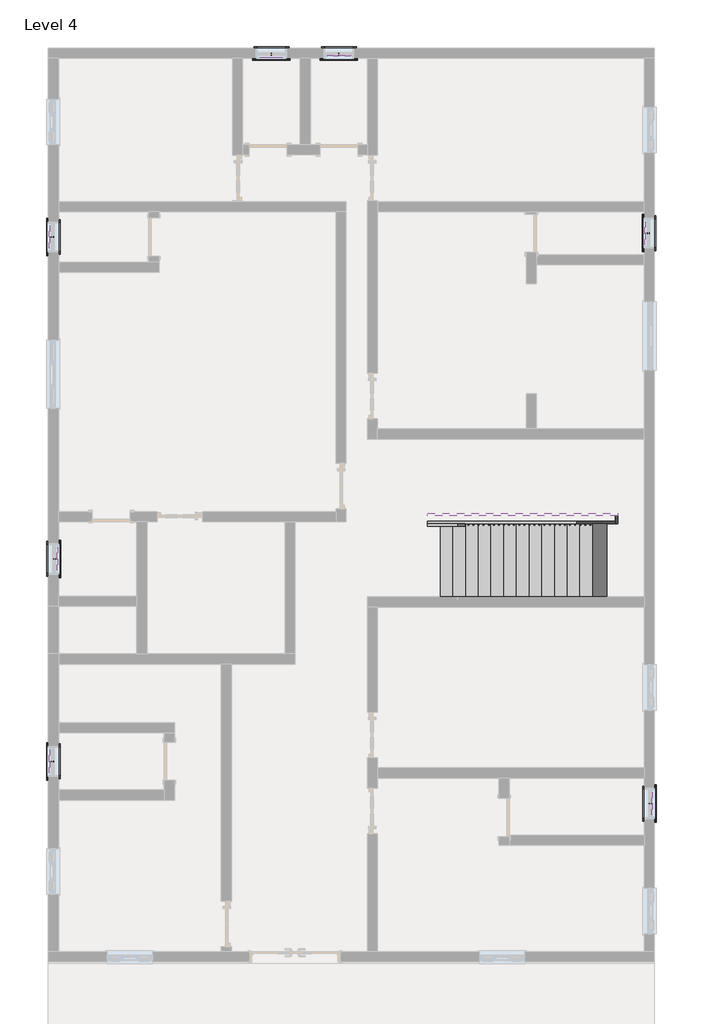
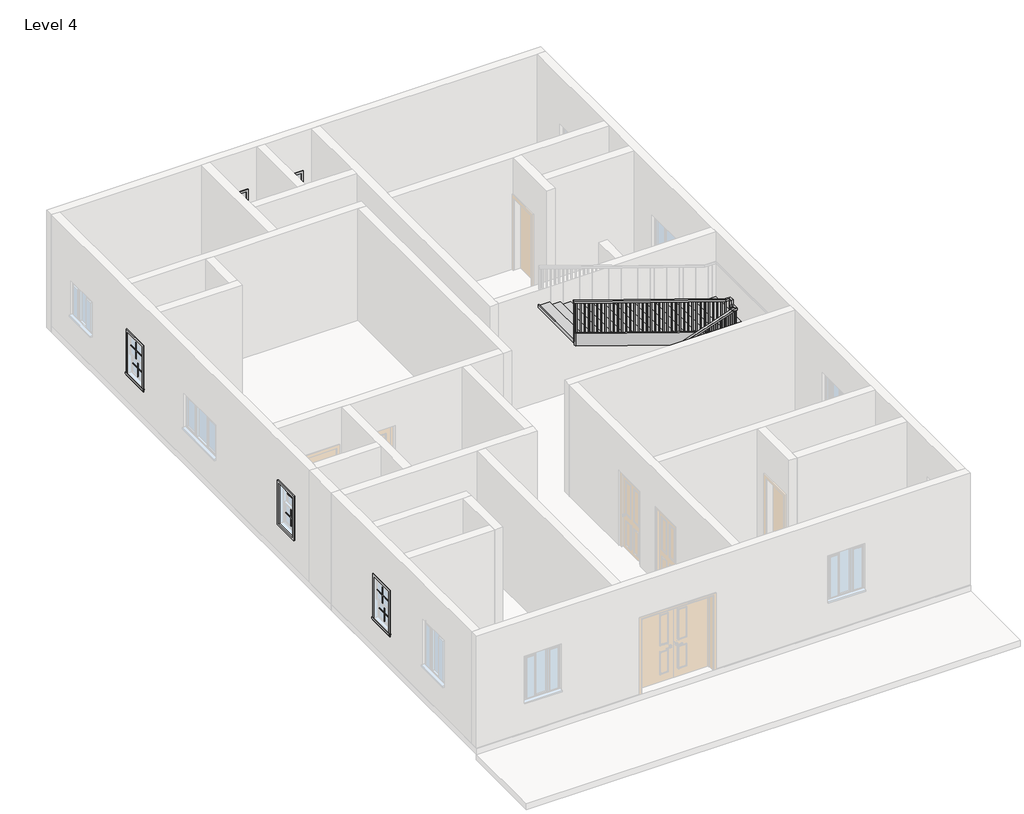
# One storey, part 3 of 3: 28 proxies, 6 members, 1 railing, 1 stair flight.
"""IFC4 building model written with IfcOpenShell, lengths in millimetres."""

from ifc_helpers import new_model, si_unit, frame, origin, place, context, project, spatial, polyline, outline, extrude, faceted_brep, transform, mapped, element, save
from components import muntin_pattern_2x2_muntin_pattern_2x2_eba6c5fb, trim_window_exterior_flat_with_sill_278e6a94, trim_window_interior_flat_picture_frame_e9fd5f45, stair_flight_fd3cf4e0

model = new_model("IFC4")

# Units and contexts
model_context = context("Model", 3, world=origin())
ifc_project = project(units=[si_unit("LENGTHUNIT", "METRE", prefix="MILLI")], contexts=[model_context])

# Site, building, storey
site = spatial("IfcSite", under=ifc_project)
building = spatial("IfcBuilding", under=site)
storey = spatial("IfcBuildingStorey", under=building, Name="Level 4", Elevation=9144.0)

# Proxies
placement = place(None, origin())
muntin_pattern_2x2_muntin_pattern_2x2_shape = muntin_pattern_2x2_muntin_pattern_2x2_eba6c5fb(model_context)
element("IfcBuildingElementProxy", 1, Name="Muntin Pattern_2x2 : Muntin Pattern_2x2", ObjectType="Muntin Pattern_2x2 : Muntin Pattern_2x2", at=placement, inside=storey, context=model_context, shape_type="MappedRepresentation", body=[
    mapped(muntin_pattern_2x2_muntin_pattern_2x2_shape, transform((-6096.8589448, 5183.1303322, 10614.025), x_axis=(0.0, 1.0, 0.0), y_axis=(-1.0, 0.0, 0.0), z_axis=(0.0, 0.0, 1.0))),
])
element("IfcBuildingElementProxy", 2, Name="Muntin Pattern_2x2 : Muntin Pattern_2x2", ObjectType="Muntin Pattern_2x2 : Muntin Pattern_2x2", at=placement, inside=storey, context=model_context, shape_type="MappedRepresentation", body=[
    mapped(muntin_pattern_2x2_muntin_pattern_2x2_shape, transform((-6052.4089448, 5183.1303322, 10134.6), x_axis=(0.0, 1.0, 0.0), y_axis=(-1.0, 0.0, 0.0), z_axis=(0.0, 0.0, 1.0))),
])
element("IfcBuildingElementProxy", 3, Name="Muntin Pattern_2x2 : Muntin Pattern_2x2", ObjectType="Muntin Pattern_2x2 : Muntin Pattern_2x2", at=placement, inside=storey, context=model_context, shape_type="MappedRepresentation", body=[
    mapped(muntin_pattern_2x2_muntin_pattern_2x2_shape, transform((-1673.5309118, 8787.5224079, 10614.025), x_axis=(-1.0, 0.0, 0.0), y_axis=(0.0, -1.0, 0.0), z_axis=(0.0, 0.0, 1.0))),
])
element("IfcBuildingElementProxy", 4, Name="Muntin Pattern_2x2 : Muntin Pattern_2x2", ObjectType="Muntin Pattern_2x2 : Muntin Pattern_2x2", at=placement, inside=storey, context=model_context, shape_type="MappedRepresentation", body=[
    mapped(muntin_pattern_2x2_muntin_pattern_2x2_shape, transform((-1673.5309118, 8831.9724079, 10134.6), x_axis=(-1.0, 0.0, 0.0), y_axis=(0.0, -1.0, 0.0), z_axis=(0.0, 0.0, 1.0))),
])
element("IfcBuildingElementProxy", 5, Name="Muntin Pattern_2x2 : Muntin Pattern_2x2", ObjectType="Muntin Pattern_2x2 : Muntin Pattern_2x2", at=placement, inside=storey, context=model_context, shape_type="MappedRepresentation", body=[
    mapped(muntin_pattern_2x2_muntin_pattern_2x2_shape, transform((-324.5451949, 8787.5224079, 10614.025), x_axis=(-1.0, 0.0, 0.0), y_axis=(0.0, -1.0, 0.0), z_axis=(0.0, 0.0, 1.0))),
])
element("IfcBuildingElementProxy", 6, Name="Muntin Pattern_2x2 : Muntin Pattern_2x2", ObjectType="Muntin Pattern_2x2 : Muntin Pattern_2x2", at=placement, inside=storey, context=model_context, shape_type="MappedRepresentation", body=[
    mapped(muntin_pattern_2x2_muntin_pattern_2x2_shape, transform((-324.5451949, 8831.9724079, 10134.6), x_axis=(-1.0, 0.0, 0.0), y_axis=(0.0, -1.0, 0.0), z_axis=(0.0, 0.0, 1.0))),
])
element("IfcBuildingElementProxy", 7, Name="Muntin Pattern_2x2 : Muntin Pattern_2x2", ObjectType="Muntin Pattern_2x2 : Muntin Pattern_2x2", at=placement, inside=storey, context=model_context, shape_type="MappedRepresentation", body=[
    mapped(muntin_pattern_2x2_muntin_pattern_2x2_shape, transform((5813.4689795, 5259.3303322, 10614.025), x_axis=(0.0, 1.0, 0.0), y_axis=(-1.0, 0.0, 0.0), z_axis=(0.0, 0.0, 1.0))),
])
element("IfcBuildingElementProxy", 8, Name="Muntin Pattern_2x2 : Muntin Pattern_2x2", ObjectType="Muntin Pattern_2x2 : Muntin Pattern_2x2", at=placement, inside=storey, context=model_context, shape_type="MappedRepresentation", body=[
    mapped(muntin_pattern_2x2_muntin_pattern_2x2_shape, transform((5857.9189795, 5259.3303322, 10134.6), x_axis=(0.0, 1.0, 0.0), y_axis=(-1.0, 0.0, 0.0), z_axis=(0.0, 0.0, 1.0))),
])
element("IfcBuildingElementProxy", 9, Name="Muntin Pattern_2x2 : Muntin Pattern_2x2", ObjectType="Muntin Pattern_2x2 : Muntin Pattern_2x2", at=placement, inside=storey, context=model_context, shape_type="MappedRepresentation", body=[
    mapped(muntin_pattern_2x2_muntin_pattern_2x2_shape, transform((5946.8189795, -6133.2488489, 10614.025), x_axis=(0.0, -1.0, 0.0), y_axis=(1.0, 0.0, 0.0), z_axis=(0.0, 0.0, 1.0))),
])
element("IfcBuildingElementProxy", 10, Name="Muntin Pattern_2x2 : Muntin Pattern_2x2", ObjectType="Muntin Pattern_2x2 : Muntin Pattern_2x2", at=placement, inside=storey, context=model_context, shape_type="MappedRepresentation", body=[
    mapped(muntin_pattern_2x2_muntin_pattern_2x2_shape, transform((5902.3689795, -6133.2488489, 10134.6), x_axis=(0.0, -1.0, 0.0), y_axis=(1.0, 0.0, 0.0), z_axis=(0.0, 0.0, 1.0))),
])
element("IfcBuildingElementProxy", 11, Name="Muntin Pattern_2x2 : Muntin Pattern_2x2", ObjectType="Muntin Pattern_2x2 : Muntin Pattern_2x2", at=placement, inside=storey, context=model_context, shape_type="MappedRepresentation", body=[
    mapped(muntin_pattern_2x2_muntin_pattern_2x2_shape, transform((-6096.8589448, -5291.0659014, 10614.025), x_axis=(0.0, 1.0, 0.0), y_axis=(-1.0, 0.0, 0.0), z_axis=(0.0, 0.0, 1.0))),
])
element("IfcBuildingElementProxy", 12, Name="Muntin Pattern_2x2 : Muntin Pattern_2x2", ObjectType="Muntin Pattern_2x2 : Muntin Pattern_2x2", at=placement, inside=storey, context=model_context, shape_type="MappedRepresentation", body=[
    mapped(muntin_pattern_2x2_muntin_pattern_2x2_shape, transform((-6052.4089448, -5291.0659014, 10134.6), x_axis=(0.0, 1.0, 0.0), y_axis=(-1.0, 0.0, 0.0), z_axis=(0.0, 0.0, 1.0))),
])
element("IfcBuildingElementProxy", 13, Name="Muntin Pattern_2x2 : Muntin Pattern_2x2", ObjectType="Muntin Pattern_2x2 : Muntin Pattern_2x2", at=placement, inside=storey, context=model_context, shape_type="MappedRepresentation", body=[
    mapped(muntin_pattern_2x2_muntin_pattern_2x2_shape, transform((-5963.5089448, -1246.1159014, 10614.025), x_axis=(0.0, -1.0, 0.0), y_axis=(1.0, 0.0, 0.0), z_axis=(0.0, 0.0, 1.0))),
])
element("IfcBuildingElementProxy", 14, Name="Muntin Pattern_2x2 : Muntin Pattern_2x2", ObjectType="Muntin Pattern_2x2 : Muntin Pattern_2x2", at=placement, inside=storey, context=model_context, shape_type="MappedRepresentation", body=[
    mapped(muntin_pattern_2x2_muntin_pattern_2x2_shape, transform((-6007.9589448, -1246.1159014, 10134.6), x_axis=(0.0, -1.0, 0.0), y_axis=(1.0, 0.0, 0.0), z_axis=(0.0, 0.0, 1.0))),
])
trim_window_exterior_flat_with_sill_shape = trim_window_exterior_flat_with_sill_278e6a94(model_context)
element("IfcBuildingElementProxy", 15, Name="Trim-Window-Exterior-Flat : with Sill", ObjectType="Trim-Window-Exterior-Flat : with Sill", at=placement, inside=storey, context=model_context, shape_type="MappedRepresentation", body=[
    mapped(trim_window_exterior_flat_with_sill_shape, transform((-6131.7839448, 5183.1303322, 11125.2), x_axis=(0.0, -1.0, 0.0), y_axis=(0.0, 0.0, 1.0), z_axis=(-1.0, 0.0, 0.0))),
])
element("IfcBuildingElementProxy", 16, Name="Trim-Window-Exterior-Flat : with Sill", ObjectType="Trim-Window-Exterior-Flat : with Sill", at=placement, inside=storey, context=model_context, shape_type="MappedRepresentation", body=[
    mapped(trim_window_exterior_flat_with_sill_shape, transform((-1673.5309118, 8752.5974079, 11125.2), x_axis=(1.0, 0.0, 0.0), y_axis=(0.0, 0.0, 1.0), z_axis=(0.0, -1.0, 0.0))),
])
element("IfcBuildingElementProxy", 17, Name="Trim-Window-Exterior-Flat : with Sill", ObjectType="Trim-Window-Exterior-Flat : with Sill", at=placement, inside=storey, context=model_context, shape_type="MappedRepresentation", body=[
    mapped(trim_window_exterior_flat_with_sill_shape, transform((-324.5451949, 8752.5974079, 11125.2), x_axis=(1.0, 0.0, 0.0), y_axis=(0.0, 0.0, 1.0), z_axis=(0.0, -1.0, 0.0))),
])
element("IfcBuildingElementProxy", 18, Name="Trim-Window-Exterior-Flat : with Sill", ObjectType="Trim-Window-Exterior-Flat : with Sill", at=placement, inside=storey, context=model_context, shape_type="MappedRepresentation", body=[
    mapped(trim_window_exterior_flat_with_sill_shape, transform((5778.5439795, 5259.3303322, 11125.2), x_axis=(0.0, -1.0, 0.0), y_axis=(0.0, 0.0, 1.0), z_axis=(-1.0, 0.0, 0.0))),
])
element("IfcBuildingElementProxy", 19, Name="Trim-Window-Exterior-Flat : with Sill", ObjectType="Trim-Window-Exterior-Flat : with Sill", at=placement, inside=storey, context=model_context, shape_type="MappedRepresentation", body=[
    mapped(trim_window_exterior_flat_with_sill_shape, transform((5981.7439795, -6133.2488489, 11125.2), x_axis=(0.0, 1.0, 0.0), y_axis=(0.0, 0.0, 1.0), z_axis=(1.0, 0.0, 0.0))),
])
element("IfcBuildingElementProxy", 20, Name="Trim-Window-Exterior-Flat : with Sill", ObjectType="Trim-Window-Exterior-Flat : with Sill", at=placement, inside=storey, context=model_context, shape_type="MappedRepresentation", body=[
    mapped(trim_window_exterior_flat_with_sill_shape, transform((-6131.7839448, -5291.0659014, 11125.2), x_axis=(0.0, -1.0, 0.0), y_axis=(0.0, 0.0, 1.0), z_axis=(-1.0, 0.0, 0.0))),
])
element("IfcBuildingElementProxy", 21, Name="Trim-Window-Exterior-Flat : with Sill", ObjectType="Trim-Window-Exterior-Flat : with Sill", at=placement, inside=storey, context=model_context, shape_type="MappedRepresentation", body=[
    mapped(trim_window_exterior_flat_with_sill_shape, transform((-5928.5839448, -1246.1159014, 11125.2), x_axis=(0.0, 1.0, 0.0), y_axis=(0.0, 0.0, 1.0), z_axis=(1.0, 0.0, 0.0))),
])
trim_window_interior_flat_picture_frame_shape = trim_window_interior_flat_picture_frame_e9fd5f45(model_context)
element("IfcBuildingElementProxy", 22, Name="Trim-Window-Interior-Flat : Picture Frame", ObjectType="Trim-Window-Interior-Flat : Picture Frame", at=placement, inside=storey, context=model_context, shape_type="MappedRepresentation", body=[
    mapped(trim_window_interior_flat_picture_frame_shape, transform((-5928.5839448, 5183.1303322, 11125.2), x_axis=(0.0, 1.0, 0.0), y_axis=(0.0, 0.0, 1.0), z_axis=(1.0, 0.0, 0.0))),
])
element("IfcBuildingElementProxy", 23, Name="Trim-Window-Interior-Flat : Picture Frame", ObjectType="Trim-Window-Interior-Flat : Picture Frame", at=placement, inside=storey, context=model_context, shape_type="MappedRepresentation", body=[
    mapped(trim_window_interior_flat_picture_frame_shape, transform((-1673.5309118, 8955.7974079, 11125.2), x_axis=(-1.0, 0.0, 0.0), y_axis=(0.0, 0.0, 1.0), z_axis=(0.0, 1.0, 0.0))),
])
element("IfcBuildingElementProxy", 24, Name="Trim-Window-Interior-Flat : Picture Frame", ObjectType="Trim-Window-Interior-Flat : Picture Frame", at=placement, inside=storey, context=model_context, shape_type="MappedRepresentation", body=[
    mapped(trim_window_interior_flat_picture_frame_shape, transform((-324.5451949, 8955.7974079, 11125.2), x_axis=(-1.0, 0.0, 0.0), y_axis=(0.0, 0.0, 1.0), z_axis=(0.0, 1.0, 0.0))),
])
element("IfcBuildingElementProxy", 25, Name="Trim-Window-Interior-Flat : Picture Frame", ObjectType="Trim-Window-Interior-Flat : Picture Frame", at=placement, inside=storey, context=model_context, shape_type="MappedRepresentation", body=[
    mapped(trim_window_interior_flat_picture_frame_shape, transform((5981.7439795, 5259.3303322, 11125.2), x_axis=(0.0, 1.0, 0.0), y_axis=(0.0, 0.0, 1.0), z_axis=(1.0, 0.0, 0.0))),
])
element("IfcBuildingElementProxy", 26, Name="Trim-Window-Interior-Flat : Picture Frame", ObjectType="Trim-Window-Interior-Flat : Picture Frame", at=placement, inside=storey, context=model_context, shape_type="MappedRepresentation", body=[
    mapped(trim_window_interior_flat_picture_frame_shape, transform((5778.5439795, -6133.2488489, 11125.2), x_axis=(0.0, -1.0, 0.0), y_axis=(0.0, 0.0, 1.0), z_axis=(-1.0, 0.0, 0.0))),
])
element("IfcBuildingElementProxy", 27, Name="Trim-Window-Interior-Flat : Picture Frame", ObjectType="Trim-Window-Interior-Flat : Picture Frame", at=placement, inside=storey, context=model_context, shape_type="MappedRepresentation", body=[
    mapped(trim_window_interior_flat_picture_frame_shape, transform((-5928.5839448, -5291.0659014, 11125.2), x_axis=(0.0, 1.0, 0.0), y_axis=(0.0, 0.0, 1.0), z_axis=(1.0, 0.0, 0.0))),
])
element("IfcBuildingElementProxy", 28, Name="Trim-Window-Interior-Flat : Picture Frame", ObjectType="Trim-Window-Interior-Flat : Picture Frame", at=placement, inside=storey, context=model_context, shape_type="MappedRepresentation", body=[
    mapped(trim_window_interior_flat_picture_frame_shape, transform((-6131.7839448, -1246.1159014, 11125.2), x_axis=(0.0, -1.0, 0.0), y_axis=(0.0, 0.0, 1.0), z_axis=(-1.0, 0.0, 0.0))),
])

# Members
element("IfcMember", 29, ObjectType="Stringer - 2\" Width", at=placement, inside=storey, context=model_context, shape_type="SweptSolid", body=[
    extrude(outline(polyline([(9337.7751932, 1449.3932247), (9144.0, 1449.3932247), (9144.0, 1827.5890963), (10284.094539, 5195.8669505), (10591.8, 5195.8669505), (10591.8, 5154.2649181), (9337.7751932, 1449.3932247)])), frame((0.0, -541.2659014, 0.0), z_axis=(0.0, 1.0, 0.0), x_axis=(0.0, 0.0, 1.0)), (0.0, 0.0, 1.0), 50.8),
])
element("IfcMember", 30, ObjectType="Stringer - 2\" Width", at=placement, inside=storey, context=model_context, shape_type="SweptSolid", body=[
    extrude(outline(polyline([(5246.6669505, -541.2659014), (5195.8669505, -541.2659014), (5195.8669505, -388.7910016), (5246.6669505, -388.7910016), (5246.6669505, -541.2659014)])), frame((0.0, 0.0, 10287.0), z_axis=(0.0, 0.0, 1.0), x_axis=(1.0, 0.0, 0.0)), (0.0, 0.0, 1.0), 304.8),
])
element("IfcMember", 31, ObjectType="Stringer - 2\" Width", at=placement, inside=storey, context=model_context, shape_type="SweptSolid", body=[
    extrude(outline(polyline([(10387.0143208, 5246.6669505), (10708.8012358, 5246.6669505), (11994.1022784, 1449.3932247), (11672.3153634, 1449.3932247), (10387.0143208, 5246.6669505)])), frame((0.0, -388.7910016, 0.0), z_axis=(0.0, 1.0, 0.0), x_axis=(0.0, 0.0, 1.0)), (0.0, 0.0, 1.0), 50.8),
])
element("IfcMember", 32, ObjectType="Stringer - 2\" Width", at=placement, inside=storey, context=model_context, shape_type="SweptSolid", body=[
    extrude(outline(polyline([(9337.7751932, 1449.3932247), (9144.0, 1449.3932247), (9144.0, 1827.5890963), (10496.1142723, 5822.2548051), (10591.8, 5822.2548051), (10591.8, 5154.2649181), (9337.7751932, 1449.3932247)])), frame((0.0, -2116.0659014, 0.0), z_axis=(0.0, 1.0, 0.0), x_axis=(0.0, 0.0, 1.0)), (0.0, 0.0, 1.0), 50.8),
])
element("IfcMember", 33, ObjectType="Stringer - 2\" Width", at=placement, inside=storey, context=model_context, shape_type="SweptSolid", body=[
    extrude(outline(polyline([(5873.0548051, -2116.0659014), (5822.2548051, -2116.0659014), (5822.2548051, 1185.9340986), (5873.0548051, 1185.9340986), (5873.0548051, -2116.0659014)])), frame((0.0, 0.0, 10287.0), z_axis=(0.0, 0.0, 1.0), x_axis=(1.0, 0.0, 0.0)), (0.0, 0.0, 1.0), 304.8),
])
element("IfcMember", 34, ObjectType="Stringer - 2\" Width", at=placement, inside=storey, context=model_context, shape_type="SweptSolid", body=[
    extrude(outline(polyline([(10287.0, 5873.0548051), (10496.7815025, 5873.0548051), (11994.1022784, 1449.3932247), (11672.3153634, 1449.3932247), (10287.0, 5542.1477288), (10287.0, 5873.0548051)])), frame((0.0, 1185.9340986, 0.0), z_axis=(0.0, 1.0, 0.0), x_axis=(0.0, 0.0, 1.0)), (0.0, 0.0, 1.0), 50.8),
])

# Railing
element("IfcRailing", 35, ObjectType="Handrail - Rectangular", at=placement, inside=storey, context=model_context, shape_type="SolidModel", body=[
    faceted_brep([(1449.3932247, -541.2659014, 10144.125), (1449.3932247, -541.2659014, 10090.4913852), (1449.3932247, -592.0659014, 10090.4913852), (1449.3932247, -592.0659014, 10144.125), (5170.4669505, -541.2659014, 11404.1963098), (5221.2669505, -541.2659014, 11367.7651551), (5221.2669505, -592.0659014, 11367.7651551), (5170.4669505, -592.0659014, 11404.1963098), (5170.4669505, -541.2659014, 11430.0), (5221.2669505, -541.2659014, 11379.2), (5221.2669505, -592.0659014, 11379.2), (5170.4669505, -592.0659014, 11430.0), (5246.6669505, -541.2659014, 11430.0), (5246.6669505, -541.2659014, 11379.2), (5297.4669505, -592.0659014, 11379.2), (5297.4669505, -592.0659014, 11430.0), (5246.6669505, -465.0659014, 11430.0), (5246.6669505, -465.0659014, 11379.2), (5297.4669505, -465.0659014, 11379.2), (5297.4669505, -465.0659014, 11430.0), (5246.6669505, -414.1910016, 11430.0), (5246.6669505, -363.3910016, 11379.2), (5297.4669505, -363.3910016, 11379.2), (5297.4669505, -414.1910016, 11430.0), (5246.6669505, -414.1910016, 11541.5286902), (5246.6669505, -363.3910016, 11490.7286902), (5297.4669505, -363.3910016, 11490.7286902), (5297.4669505, -414.1910016, 11541.5286902), (5246.6669505, -337.9910016, 11541.5286902), (5246.6669505, -337.9910016, 11490.7286902), (5297.4669505, -287.1910016, 11490.7286902), (5297.4669505, -287.1910016, 11541.5286902), (5170.4669505, -337.9910016, 11541.5286902), (5162.099099, -337.9910016, 11490.7286902), (5162.099099, -287.1910016, 11490.7286902), (5170.4669505, -287.1910016, 11541.5286902), (1449.3932247, -337.9910016, 12801.6), (1449.3932247, -287.1910016, 12801.6), (1449.3932247, -287.1910016, 12747.9663852), (1449.3932247, -337.9910016, 12747.9663852)], [[[0, 1, 2, 3]], [[1, 0, 4, 5]], [[2, 1, 5, 6]], [[3, 2, 6, 7]], [[0, 3, 7, 4]], [[5, 4, 8, 9]], [[6, 5, 9, 10]], [[7, 6, 10, 11]], [[4, 7, 11, 8]], [[9, 8, 12, 13]], [[10, 9, 13, 14]], [[11, 10, 14, 15]], [[8, 11, 15, 12]], [[13, 12, 16, 17]], [[14, 13, 17, 18]], [[15, 14, 18, 19]], [[12, 15, 19, 16]], [[17, 16, 20, 21]], [[18, 17, 21, 22]], [[19, 18, 22, 23]], [[16, 19, 23, 20]], [[21, 20, 24, 25]], [[22, 21, 25, 26]], [[23, 22, 26, 27]], [[20, 23, 27, 24]], [[25, 24, 28, 29]], [[26, 25, 29, 30]], [[27, 26, 30, 31]], [[24, 27, 31, 28]], [[29, 28, 32, 33]], [[30, 29, 33, 34]], [[31, 30, 34, 35]], [[28, 31, 35, 32]], [[36, 37, 38, 39]], [[33, 32, 36, 39]], [[34, 33, 39, 38]], [[35, 34, 38, 37]], [[32, 35, 37, 36]]]),
    extrude(outline(polyline([(12729.6976686, 1503.3419505), (11801.475, 1503.3419505), (11801.475, 1522.3919505), (12723.246746, 1522.3919505), (12729.6976686, 1503.3419505)])), frame((0.0, -322.1160016, 0.0), z_axis=(0.0, 1.0, 0.0), x_axis=(0.0, 0.0, 1.0)), (0.0, 0.0, 1.0), 19.05),
    extrude(outline(polyline([(12695.2927482, 1604.9419505), (11801.475, 1604.9419505), (11801.475, 1623.9919505), (12688.8418257, 1623.9919505), (12695.2927482, 1604.9419505)])), frame((0.0, -322.1160016, 0.0), z_axis=(0.0, 1.0, 0.0), x_axis=(0.0, 0.0, 1.0)), (0.0, 0.0, 1.0), 19.05),
    extrude(outline(polyline([(12660.8878279, 1706.5419505), (11715.75, 1706.5419505), (11715.75, 1725.5919505), (12654.4369054, 1725.5919505), (12660.8878279, 1706.5419505)])), frame((0.0, -322.1160016, 0.0), z_axis=(0.0, 1.0, 0.0), x_axis=(0.0, 0.0, 1.0)), (0.0, 0.0, 1.0), 19.05),
    extrude(outline(polyline([(12626.4829076, 1808.1419505), (11715.75, 1808.1419505), (11715.75, 1827.1919505), (12620.031985, 1827.1919505), (12626.4829076, 1808.1419505)])), frame((0.0, -322.1160016, 0.0), z_axis=(0.0, 1.0, 0.0), x_axis=(0.0, 0.0, 1.0)), (0.0, 0.0, 1.0), 19.05),
    extrude(outline(polyline([(12592.0779873, 1909.7419505), (11715.75, 1909.7419505), (11715.75, 1928.7919505), (12585.6270647, 1928.7919505), (12592.0779873, 1909.7419505)])), frame((0.0, -322.1160016, 0.0), z_axis=(0.0, 1.0, 0.0), x_axis=(0.0, 0.0, 1.0)), (0.0, 0.0, 1.0), 19.05),
    extrude(outline(polyline([(12557.6730669, 2011.3419505), (11630.025, 2011.3419505), (11630.025, 2030.3919505), (12551.2221444, 2030.3919505), (12557.6730669, 2011.3419505)])), frame((0.0, -322.1160016, 0.0), z_axis=(0.0, 1.0, 0.0), x_axis=(0.0, 0.0, 1.0)), (0.0, 0.0, 1.0), 19.05),
    extrude(outline(polyline([(12523.2681466, 2112.9419505), (11630.025, 2112.9419505), (11630.025, 2131.9919505), (12516.817224, 2131.9919505), (12523.2681466, 2112.9419505)])), frame((0.0, -322.1160016, 0.0), z_axis=(0.0, 1.0, 0.0), x_axis=(0.0, 0.0, 1.0)), (0.0, 0.0, 1.0), 19.05),
    extrude(outline(polyline([(12488.8632263, 2214.5419505), (11544.3, 2214.5419505), (11544.3, 2233.5919505), (12482.4123037, 2233.5919505), (12488.8632263, 2214.5419505)])), frame((0.0, -322.1160016, 0.0), z_axis=(0.0, 1.0, 0.0), x_axis=(0.0, 0.0, 1.0)), (0.0, 0.0, 1.0), 19.05),
    extrude(outline(polyline([(12454.4583059, 2316.1419505), (11544.3, 2316.1419505), (11544.3, 2335.1919505), (12448.0073834, 2335.1919505), (12454.4583059, 2316.1419505)])), frame((0.0, -322.1160016, 0.0), z_axis=(0.0, 1.0, 0.0), x_axis=(0.0, 0.0, 1.0)), (0.0, 0.0, 1.0), 19.05),
    extrude(outline(polyline([(12420.0533856, 2417.7419505), (11544.3, 2417.7419505), (11544.3, 2436.7919505), (12413.6024631, 2436.7919505), (12420.0533856, 2417.7419505)])), frame((0.0, -322.1160016, 0.0), z_axis=(0.0, 1.0, 0.0), x_axis=(0.0, 0.0, 1.0)), (0.0, 0.0, 1.0), 19.05),
    extrude(outline(polyline([(12385.6484653, 2519.3419505), (11458.575, 2519.3419505), (11458.575, 2538.3919505), (12379.1975427, 2538.3919505), (12385.6484653, 2519.3419505)])), frame((0.0, -322.1160016, 0.0), z_axis=(0.0, 1.0, 0.0), x_axis=(0.0, 0.0, 1.0)), (0.0, 0.0, 1.0), 19.05),
    extrude(outline(polyline([(12351.243545, 2620.9419505), (11458.575, 2620.9419505), (11458.575, 2639.9919505), (12344.7926224, 2639.9919505), (12351.243545, 2620.9419505)])), frame((0.0, -322.1160016, 0.0), z_axis=(0.0, 1.0, 0.0), x_axis=(0.0, 0.0, 1.0)), (0.0, 0.0, 1.0), 19.05),
    extrude(outline(polyline([(12316.8386246, 2722.5419505), (11372.85, 2722.5419505), (11372.85, 2741.5919505), (12310.3877021, 2741.5919505), (12316.8386246, 2722.5419505)])), frame((0.0, -322.1160016, 0.0), z_axis=(0.0, 1.0, 0.0), x_axis=(0.0, 0.0, 1.0)), (0.0, 0.0, 1.0), 19.05),
    extrude(outline(polyline([(12282.4337043, 2824.1419505), (11372.85, 2824.1419505), (11372.85, 2843.1919505), (12275.9827817, 2843.1919505), (12282.4337043, 2824.1419505)])), frame((0.0, -322.1160016, 0.0), z_axis=(0.0, 1.0, 0.0), x_axis=(0.0, 0.0, 1.0)), (0.0, 0.0, 1.0), 19.05),
    extrude(outline(polyline([(12248.028784, 2925.7419505), (11372.85, 2925.7419505), (11372.85, 2944.7919505), (12241.5778614, 2944.7919505), (12248.028784, 2925.7419505)])), frame((0.0, -322.1160016, 0.0), z_axis=(0.0, 1.0, 0.0), x_axis=(0.0, 0.0, 1.0)), (0.0, 0.0, 1.0), 19.05),
    extrude(outline(polyline([(12213.6238636, 3027.3419505), (11287.125, 3027.3419505), (11287.125, 3046.3919505), (12207.1729411, 3046.3919505), (12213.6238636, 3027.3419505)])), frame((0.0, -322.1160016, 0.0), z_axis=(0.0, 1.0, 0.0), x_axis=(0.0, 0.0, 1.0)), (0.0, 0.0, 1.0), 19.05),
    extrude(outline(polyline([(12179.2189433, 3128.9419505), (11287.125, 3128.9419505), (11287.125, 3147.9919505), (12172.7680208, 3147.9919505), (12179.2189433, 3128.9419505)])), frame((0.0, -322.1160016, 0.0), z_axis=(0.0, 1.0, 0.0), x_axis=(0.0, 0.0, 1.0)), (0.0, 0.0, 1.0), 19.05),
    extrude(outline(polyline([(12144.814023, 3230.5419505), (11201.4, 3230.5419505), (11201.4, 3249.5919505), (12138.3631004, 3249.5919505), (12144.814023, 3230.5419505)])), frame((0.0, -322.1160016, 0.0), z_axis=(0.0, 1.0, 0.0), x_axis=(0.0, 0.0, 1.0)), (0.0, 0.0, 1.0), 19.05),
    extrude(outline(polyline([(12110.4091027, 3332.1419505), (11201.4, 3332.1419505), (11201.4, 3351.1919505), (12103.9581801, 3351.1919505), (12110.4091027, 3332.1419505)])), frame((0.0, -322.1160016, 0.0), z_axis=(0.0, 1.0, 0.0), x_axis=(0.0, 0.0, 1.0)), (0.0, 0.0, 1.0), 19.05),
    extrude(outline(polyline([(12076.0041823, 3433.7419505), (11201.4, 3433.7419505), (11201.4, 3452.7919505), (12069.5532598, 3452.7919505), (12076.0041823, 3433.7419505)])), frame((0.0, -322.1160016, 0.0), z_axis=(0.0, 1.0, 0.0), x_axis=(0.0, 0.0, 1.0)), (0.0, 0.0, 1.0), 19.05),
    extrude(outline(polyline([(12041.599262, 3535.3419505), (11115.675, 3535.3419505), (11115.675, 3554.3919505), (12035.1483394, 3554.3919505), (12041.599262, 3535.3419505)])), frame((0.0, -322.1160016, 0.0), z_axis=(0.0, 1.0, 0.0), x_axis=(0.0, 0.0, 1.0)), (0.0, 0.0, 1.0), 19.05),
    extrude(outline(polyline([(12007.1943417, 3636.9419505), (11115.675, 3636.9419505), (11115.675, 3655.9919505), (12000.7434191, 3655.9919505), (12007.1943417, 3636.9419505)])), frame((0.0, -322.1160016, 0.0), z_axis=(0.0, 1.0, 0.0), x_axis=(0.0, 0.0, 1.0)), (0.0, 0.0, 1.0), 19.05),
    extrude(outline(polyline([(11972.7894213, 3738.5419505), (11029.95, 3738.5419505), (11029.95, 3757.5919505), (11966.3384988, 3757.5919505), (11972.7894213, 3738.5419505)])), frame((0.0, -322.1160016, 0.0), z_axis=(0.0, 1.0, 0.0), x_axis=(0.0, 0.0, 1.0)), (0.0, 0.0, 1.0), 19.05),
    extrude(outline(polyline([(11938.384501, 3840.1419505), (11029.95, 3840.1419505), (11029.95, 3859.1919505), (11931.9335784, 3859.1919505), (11938.384501, 3840.1419505)])), frame((0.0, -322.1160016, 0.0), z_axis=(0.0, 1.0, 0.0), x_axis=(0.0, 0.0, 1.0)), (0.0, 0.0, 1.0), 19.05),
    extrude(outline(polyline([(11903.9795807, 3941.7419505), (11029.95, 3941.7419505), (11029.95, 3960.7919505), (11897.5286581, 3960.7919505), (11903.9795807, 3941.7419505)])), frame((0.0, -322.1160016, 0.0), z_axis=(0.0, 1.0, 0.0), x_axis=(0.0, 0.0, 1.0)), (0.0, 0.0, 1.0), 19.05),
    extrude(outline(polyline([(11869.5746604, 4043.3419505), (10944.225, 4043.3419505), (10944.225, 4062.3919505), (11863.1237378, 4062.3919505), (11869.5746604, 4043.3419505)])), frame((0.0, -322.1160016, 0.0), z_axis=(0.0, 1.0, 0.0), x_axis=(0.0, 0.0, 1.0)), (0.0, 0.0, 1.0), 19.05),
    extrude(outline(polyline([(11835.16974, 4144.9419505), (10944.225, 4144.9419505), (10944.225, 4163.9919505), (11828.7188175, 4163.9919505), (11835.16974, 4144.9419505)])), frame((0.0, -322.1160016, 0.0), z_axis=(0.0, 1.0, 0.0), x_axis=(0.0, 0.0, 1.0)), (0.0, 0.0, 1.0), 19.05),
    extrude(outline(polyline([(11800.7648197, 4246.5419505), (10858.5, 4246.5419505), (10858.5, 4265.5919505), (11794.3138971, 4265.5919505), (11800.7648197, 4246.5419505)])), frame((0.0, -322.1160016, 0.0), z_axis=(0.0, 1.0, 0.0), x_axis=(0.0, 0.0, 1.0)), (0.0, 0.0, 1.0), 19.05),
    extrude(outline(polyline([(11766.3598994, 4348.1419505), (10858.5, 4348.1419505), (10858.5, 4367.1919505), (11759.9089768, 4367.1919505), (11766.3598994, 4348.1419505)])), frame((0.0, -322.1160016, 0.0), z_axis=(0.0, 1.0, 0.0), x_axis=(0.0, 0.0, 1.0)), (0.0, 0.0, 1.0), 19.05),
    extrude(outline(polyline([(11731.954979, 4449.7419505), (10858.5, 4449.7419505), (10858.5, 4468.7919505), (11725.5040565, 4468.7919505), (11731.954979, 4449.7419505)])), frame((0.0, -322.1160016, 0.0), z_axis=(0.0, 1.0, 0.0), x_axis=(0.0, 0.0, 1.0)), (0.0, 0.0, 1.0), 19.05),
    extrude(outline(polyline([(11697.5500587, 4551.3419505), (10772.775, 4551.3419505), (10772.775, 4570.3919505), (11691.0991361, 4570.3919505), (11697.5500587, 4551.3419505)])), frame((0.0, -322.1160016, 0.0), z_axis=(0.0, 1.0, 0.0), x_axis=(0.0, 0.0, 1.0)), (0.0, 0.0, 1.0), 19.05),
    extrude(outline(polyline([(11663.1451384, 4652.9419505), (10772.775, 4652.9419505), (10772.775, 4671.9919505), (11656.6942158, 4671.9919505), (11663.1451384, 4652.9419505)])), frame((0.0, -322.1160016, 0.0), z_axis=(0.0, 1.0, 0.0), x_axis=(0.0, 0.0, 1.0)), (0.0, 0.0, 1.0), 19.05),
    extrude(outline(polyline([(11628.7402181, 4754.5419505), (10687.05, 4754.5419505), (10687.05, 4773.5919505), (11622.2892955, 4773.5919505), (11628.7402181, 4754.5419505)])), frame((0.0, -322.1160016, 0.0), z_axis=(0.0, 1.0, 0.0), x_axis=(0.0, 0.0, 1.0)), (0.0, 0.0, 1.0), 19.05),
    extrude(outline(polyline([(11594.3352977, 4856.1419505), (10687.05, 4856.1419505), (10687.05, 4875.1919505), (11587.8843752, 4875.1919505), (11594.3352977, 4856.1419505)])), frame((0.0, -322.1160016, 0.0), z_axis=(0.0, 1.0, 0.0), x_axis=(0.0, 0.0, 1.0)), (0.0, 0.0, 1.0), 19.05),
    extrude(outline(polyline([(11559.9303774, 4957.7419505), (10687.05, 4957.7419505), (10687.05, 4976.7919505), (11553.4794548, 4976.7919505), (11559.9303774, 4957.7419505)])), frame((0.0, -322.1160016, 0.0), z_axis=(0.0, 1.0, 0.0), x_axis=(0.0, 0.0, 1.0)), (0.0, 0.0, 1.0), 19.05),
    extrude(outline(polyline([(11525.5254571, 5059.3419505), (10601.325, 5059.3419505), (10601.325, 5078.3919505), (11519.0745345, 5078.3919505), (11525.5254571, 5059.3419505)])), frame((0.0, -322.1160016, 0.0), z_axis=(0.0, 1.0, 0.0), x_axis=(0.0, 0.0, 1.0)), (0.0, 0.0, 1.0), 19.05),
    extrude(outline(polyline([(11491.1205367, 5160.9419505), (10601.325, 5160.9419505), (10601.325, 5179.9919505), (11484.6696142, 5179.9919505), (11491.1205367, 5160.9419505)])), frame((0.0, -322.1160016, 0.0), z_axis=(0.0, 1.0, 0.0), x_axis=(0.0, 0.0, 1.0)), (0.0, 0.0, 1.0), 19.05),
    extrude(outline(polyline([(5262.5419505, -372.9909014), (5262.5419505, -353.9409014), (5281.5919505, -353.9409014), (5281.5919505, -372.9909014), (5262.5419505, -372.9909014)])), frame((0.0, 0.0, 10515.6), z_axis=(0.0, 0.0, 1.0), x_axis=(1.0, 0.0, 0.0)), (0.0, 0.0, 1.0), 975.1286902),
    extrude(outline(polyline([(5262.5419505, -474.5909014), (5262.5419505, -455.5409014), (5281.5919505, -455.5409014), (5281.5919505, -474.5909014), (5262.5419505, -474.5909014)])), frame((0.0, 0.0, 10515.6), z_axis=(0.0, 0.0, 1.0), x_axis=(1.0, 0.0, 0.0)), (0.0, 0.0, 1.0), 863.6),
    extrude(outline(polyline([(5199.0682247, -557.1409014), (5218.1182247, -557.1409014), (5218.1182247, -576.1909014), (5199.0682247, -576.1909014), (5199.0682247, -557.1409014)])), frame((0.0, 0.0, 10429.875), z_axis=(0.0, 0.0, 1.0), x_axis=(1.0, 0.0, 0.0)), (0.0, 0.0, 1.0), 949.325),
    extrude(outline(polyline([(11325.8430558, 5097.4682247), (10429.875, 5097.4682247), (10429.875, 5116.5182247), (11332.2939783, 5116.5182247), (11325.8430558, 5097.4682247)])), frame((0.0, -576.1909014, 0.0), z_axis=(0.0, 1.0, 0.0), x_axis=(0.0, 0.0, 1.0)), (0.0, 0.0, 1.0), 19.05),
    extrude(outline(polyline([(11291.4381354, 4995.8682247), (10429.875, 4995.8682247), (10429.875, 5014.9182247), (11297.889058, 5014.9182247), (11291.4381354, 4995.8682247)])), frame((0.0, -576.1909014, 0.0), z_axis=(0.0, 1.0, 0.0), x_axis=(0.0, 0.0, 1.0)), (0.0, 0.0, 1.0), 19.05),
    extrude(outline(polyline([(11257.0332151, 4894.2682247), (10344.15, 4894.2682247), (10344.15, 4913.3182247), (11263.4841377, 4913.3182247), (11257.0332151, 4894.2682247)])), frame((0.0, -576.1909014, 0.0), z_axis=(0.0, 1.0, 0.0), x_axis=(0.0, 0.0, 1.0)), (0.0, 0.0, 1.0), 19.05),
    extrude(outline(polyline([(11222.6282948, 4792.6682247), (10344.15, 4792.6682247), (10344.15, 4811.7182247), (11229.0792173, 4811.7182247), (11222.6282948, 4792.6682247)])), frame((0.0, -576.1909014, 0.0), z_axis=(0.0, 1.0, 0.0), x_axis=(0.0, 0.0, 1.0)), (0.0, 0.0, 1.0), 19.05),
    extrude(outline(polyline([(11188.2233745, 4691.0682247), (10258.425, 4691.0682247), (10258.425, 4710.1182247), (11194.674297, 4710.1182247), (11188.2233745, 4691.0682247)])), frame((0.0, -576.1909014, 0.0), z_axis=(0.0, 1.0, 0.0), x_axis=(0.0, 0.0, 1.0)), (0.0, 0.0, 1.0), 19.05),
    extrude(outline(polyline([(11153.8184541, 4589.4682247), (10258.425, 4589.4682247), (10258.425, 4608.5182247), (11160.2693767, 4608.5182247), (11153.8184541, 4589.4682247)])), frame((0.0, -576.1909014, 0.0), z_axis=(0.0, 1.0, 0.0), x_axis=(0.0, 0.0, 1.0)), (0.0, 0.0, 1.0), 19.05),
    extrude(outline(polyline([(11119.4135338, 4487.8682247), (10258.425, 4487.8682247), (10258.425, 4506.9182247), (11125.8644564, 4506.9182247), (11119.4135338, 4487.8682247)])), frame((0.0, -576.1909014, 0.0), z_axis=(0.0, 1.0, 0.0), x_axis=(0.0, 0.0, 1.0)), (0.0, 0.0, 1.0), 19.05),
    extrude(outline(polyline([(11085.0086135, 4386.2682247), (10172.7, 4386.2682247), (10172.7, 4405.3182247), (11091.459536, 4405.3182247), (11085.0086135, 4386.2682247)])), frame((0.0, -576.1909014, 0.0), z_axis=(0.0, 1.0, 0.0), x_axis=(0.0, 0.0, 1.0)), (0.0, 0.0, 1.0), 19.05),
    extrude(outline(polyline([(11050.6036931, 4284.6682247), (10172.7, 4284.6682247), (10172.7, 4303.7182247), (11057.0546157, 4303.7182247), (11050.6036931, 4284.6682247)])), frame((0.0, -576.1909014, 0.0), z_axis=(0.0, 1.0, 0.0), x_axis=(0.0, 0.0, 1.0)), (0.0, 0.0, 1.0), 19.05),
    extrude(outline(polyline([(11016.1987728, 4183.0682247), (10086.975, 4183.0682247), (10086.975, 4202.1182247), (11022.6496954, 4202.1182247), (11016.1987728, 4183.0682247)])), frame((0.0, -576.1909014, 0.0), z_axis=(0.0, 1.0, 0.0), x_axis=(0.0, 0.0, 1.0)), (0.0, 0.0, 1.0), 19.05),
    extrude(outline(polyline([(10981.7938525, 4081.4682247), (10086.975, 4081.4682247), (10086.975, 4100.5182247), (10988.244775, 4100.5182247), (10981.7938525, 4081.4682247)])), frame((0.0, -576.1909014, 0.0), z_axis=(0.0, 1.0, 0.0), x_axis=(0.0, 0.0, 1.0)), (0.0, 0.0, 1.0), 19.05),
    extrude(outline(polyline([(10947.3889321, 3979.8682247), (10086.975, 3979.8682247), (10086.975, 3998.9182247), (10953.8398547, 3998.9182247), (10947.3889321, 3979.8682247)])), frame((0.0, -576.1909014, 0.0), z_axis=(0.0, 1.0, 0.0), x_axis=(0.0, 0.0, 1.0)), (0.0, 0.0, 1.0), 19.05),
    extrude(outline(polyline([(10912.9840118, 3878.2682247), (10001.25, 3878.2682247), (10001.25, 3897.3182247), (10919.4349344, 3897.3182247), (10912.9840118, 3878.2682247)])), frame((0.0, -576.1909014, 0.0), z_axis=(0.0, 1.0, 0.0), x_axis=(0.0, 0.0, 1.0)), (0.0, 0.0, 1.0), 19.05),
    extrude(outline(polyline([(10878.5790915, 3776.6682247), (10001.25, 3776.6682247), (10001.25, 3795.7182247), (10885.0300141, 3795.7182247), (10878.5790915, 3776.6682247)])), frame((0.0, -576.1909014, 0.0), z_axis=(0.0, 1.0, 0.0), x_axis=(0.0, 0.0, 1.0)), (0.0, 0.0, 1.0), 19.05),
    extrude(outline(polyline([(10844.1741712, 3675.0682247), (9915.525, 3675.0682247), (9915.525, 3694.1182247), (10850.6250937, 3694.1182247), (10844.1741712, 3675.0682247)])), frame((0.0, -576.1909014, 0.0), z_axis=(0.0, 1.0, 0.0), x_axis=(0.0, 0.0, 1.0)), (0.0, 0.0, 1.0), 19.05),
    extrude(outline(polyline([(10809.7692508, 3573.4682247), (9915.525, 3573.4682247), (9915.525, 3592.5182247), (10816.2201734, 3592.5182247), (10809.7692508, 3573.4682247)])), frame((0.0, -576.1909014, 0.0), z_axis=(0.0, 1.0, 0.0), x_axis=(0.0, 0.0, 1.0)), (0.0, 0.0, 1.0), 19.05),
    extrude(outline(polyline([(10775.3643305, 3471.8682247), (9915.525, 3471.8682247), (9915.525, 3490.9182247), (10781.8152531, 3490.9182247), (10775.3643305, 3471.8682247)])), frame((0.0, -576.1909014, 0.0), z_axis=(0.0, 1.0, 0.0), x_axis=(0.0, 0.0, 1.0)), (0.0, 0.0, 1.0), 19.05),
    extrude(outline(polyline([(10740.9594102, 3370.2682247), (9829.8, 3370.2682247), (9829.8, 3389.3182247), (10747.4103327, 3389.3182247), (10740.9594102, 3370.2682247)])), frame((0.0, -576.1909014, 0.0), z_axis=(0.0, 1.0, 0.0), x_axis=(0.0, 0.0, 1.0)), (0.0, 0.0, 1.0), 19.05),
    extrude(outline(polyline([(10706.5544898, 3268.6682247), (9829.8, 3268.6682247), (9829.8, 3287.7182247), (10713.0054124, 3287.7182247), (10706.5544898, 3268.6682247)])), frame((0.0, -576.1909014, 0.0), z_axis=(0.0, 1.0, 0.0), x_axis=(0.0, 0.0, 1.0)), (0.0, 0.0, 1.0), 19.05),
    extrude(outline(polyline([(10672.1495695, 3167.0682247), (9744.075, 3167.0682247), (9744.075, 3186.1182247), (10678.6004921, 3186.1182247), (10672.1495695, 3167.0682247)])), frame((0.0, -576.1909014, 0.0), z_axis=(0.0, 1.0, 0.0), x_axis=(0.0, 0.0, 1.0)), (0.0, 0.0, 1.0), 19.05),
    extrude(outline(polyline([(10637.7446492, 3065.4682247), (9744.075, 3065.4682247), (9744.075, 3084.5182247), (10644.1955718, 3084.5182247), (10637.7446492, 3065.4682247)])), frame((0.0, -576.1909014, 0.0), z_axis=(0.0, 1.0, 0.0), x_axis=(0.0, 0.0, 1.0)), (0.0, 0.0, 1.0), 19.05),
    extrude(outline(polyline([(10603.3397289, 2963.8682247), (9744.075, 2963.8682247), (9744.075, 2982.9182247), (10609.7906514, 2982.9182247), (10603.3397289, 2963.8682247)])), frame((0.0, -576.1909014, 0.0), z_axis=(0.0, 1.0, 0.0), x_axis=(0.0, 0.0, 1.0)), (0.0, 0.0, 1.0), 19.05),
    extrude(outline(polyline([(10568.9348085, 2862.2682247), (9658.35, 2862.2682247), (9658.35, 2881.3182247), (10575.3857311, 2881.3182247), (10568.9348085, 2862.2682247)])), frame((0.0, -576.1909014, 0.0), z_axis=(0.0, 1.0, 0.0), x_axis=(0.0, 0.0, 1.0)), (0.0, 0.0, 1.0), 19.05),
    extrude(outline(polyline([(10534.5298882, 2760.6682247), (9658.35, 2760.6682247), (9658.35, 2779.7182247), (10540.9808108, 2779.7182247), (10534.5298882, 2760.6682247)])), frame((0.0, -576.1909014, 0.0), z_axis=(0.0, 1.0, 0.0), x_axis=(0.0, 0.0, 1.0)), (0.0, 0.0, 1.0), 19.05),
    extrude(outline(polyline([(10500.1249679, 2659.0682247), (9572.625, 2659.0682247), (9572.625, 2678.1182247), (10506.5758904, 2678.1182247), (10500.1249679, 2659.0682247)])), frame((0.0, -576.1909014, 0.0), z_axis=(0.0, 1.0, 0.0), x_axis=(0.0, 0.0, 1.0)), (0.0, 0.0, 1.0), 19.05),
    extrude(outline(polyline([(10465.7200475, 2557.4682247), (9572.625, 2557.4682247), (9572.625, 2576.5182247), (10472.1709701, 2576.5182247), (10465.7200475, 2557.4682247)])), frame((0.0, -576.1909014, 0.0), z_axis=(0.0, 1.0, 0.0), x_axis=(0.0, 0.0, 1.0)), (0.0, 0.0, 1.0), 19.05),
    extrude(outline(polyline([(10431.3151272, 2455.8682247), (9572.625, 2455.8682247), (9572.625, 2474.9182247), (10437.7660498, 2474.9182247), (10431.3151272, 2455.8682247)])), frame((0.0, -576.1909014, 0.0), z_axis=(0.0, 1.0, 0.0), x_axis=(0.0, 0.0, 1.0)), (0.0, 0.0, 1.0), 19.05),
    extrude(outline(polyline([(10396.9102069, 2354.2682247), (9486.9, 2354.2682247), (9486.9, 2373.3182247), (10403.3611294, 2373.3182247), (10396.9102069, 2354.2682247)])), frame((0.0, -576.1909014, 0.0), z_axis=(0.0, 1.0, 0.0), x_axis=(0.0, 0.0, 1.0)), (0.0, 0.0, 1.0), 19.05),
    extrude(outline(polyline([(10362.5052866, 2252.6682247), (9486.9, 2252.6682247), (9486.9, 2271.7182247), (10368.9562091, 2271.7182247), (10362.5052866, 2252.6682247)])), frame((0.0, -576.1909014, 0.0), z_axis=(0.0, 1.0, 0.0), x_axis=(0.0, 0.0, 1.0)), (0.0, 0.0, 1.0), 19.05),
    extrude(outline(polyline([(10328.1003662, 2151.0682247), (9401.175, 2151.0682247), (9401.175, 2170.1182247), (10334.5512888, 2170.1182247), (10328.1003662, 2151.0682247)])), frame((0.0, -576.1909014, 0.0), z_axis=(0.0, 1.0, 0.0), x_axis=(0.0, 0.0, 1.0)), (0.0, 0.0, 1.0), 19.05),
    extrude(outline(polyline([(10293.6954459, 2049.4682247), (9401.175, 2049.4682247), (9401.175, 2068.5182247), (10300.1463685, 2068.5182247), (10293.6954459, 2049.4682247)])), frame((0.0, -576.1909014, 0.0), z_axis=(0.0, 1.0, 0.0), x_axis=(0.0, 0.0, 1.0)), (0.0, 0.0, 1.0), 19.05),
    extrude(outline(polyline([(10259.2905256, 1947.8682247), (9401.175, 1947.8682247), (9401.175, 1966.9182247), (10265.7414481, 1966.9182247), (10259.2905256, 1947.8682247)])), frame((0.0, -576.1909014, 0.0), z_axis=(0.0, 1.0, 0.0), x_axis=(0.0, 0.0, 1.0)), (0.0, 0.0, 1.0), 19.05),
    extrude(outline(polyline([(10224.8856052, 1846.2682247), (9315.45, 1846.2682247), (9315.45, 1865.3182247), (10231.3365278, 1865.3182247), (10224.8856052, 1846.2682247)])), frame((0.0, -576.1909014, 0.0), z_axis=(0.0, 1.0, 0.0), x_axis=(0.0, 0.0, 1.0)), (0.0, 0.0, 1.0), 19.05),
    extrude(outline(polyline([(10190.4806849, 1744.6682247), (9315.45, 1744.6682247), (9315.45, 1763.7182247), (10196.9316075, 1763.7182247), (10190.4806849, 1744.6682247)])), frame((0.0, -576.1909014, 0.0), z_axis=(0.0, 1.0, 0.0), x_axis=(0.0, 0.0, 1.0)), (0.0, 0.0, 1.0), 19.05),
    extrude(outline(polyline([(10156.0757646, 1643.0682247), (9229.725, 1643.0682247), (9229.725, 1662.1182247), (10162.5266871, 1662.1182247), (10156.0757646, 1643.0682247)])), frame((0.0, -576.1909014, 0.0), z_axis=(0.0, 1.0, 0.0), x_axis=(0.0, 0.0, 1.0)), (0.0, 0.0, 1.0), 19.05),
    extrude(outline(polyline([(10121.6708443, 1541.4682247), (9229.725, 1541.4682247), (9229.725, 1560.5182247), (10128.1217668, 1560.5182247), (10121.6708443, 1541.4682247)])), frame((0.0, -576.1909014, 0.0), z_axis=(0.0, 1.0, 0.0), x_axis=(0.0, 0.0, 1.0)), (0.0, 0.0, 1.0), 19.05),
    extrude(outline(polyline([(5262.5419505, -322.1160016), (5262.5419505, -303.0660016), (5281.5919505, -303.0660016), (5281.5919505, -322.1160016), (5262.5419505, -322.1160016)])), frame((0.0, 0.0, 10515.6), z_axis=(0.0, 0.0, 1.0), x_axis=(1.0, 0.0, 0.0)), (0.0, 0.0, 1.0), 975.1286902),
    extrude(outline(polyline([(5262.5419505, -557.1409014), (5281.5919505, -557.1409014), (5281.5919505, -576.1909014), (5262.5419505, -576.1909014), (5262.5419505, -557.1409014)])), frame((0.0, 0.0, 10515.6), z_axis=(0.0, 0.0, 1.0), x_axis=(1.0, 0.0, 0.0)), (0.0, 0.0, 1.0), 863.6),
    extrude(outline(polyline([(12747.9663852, 1449.3932247), (11801.475, 1449.3932247), (11801.475, 1468.4432247), (12741.5154626, 1468.4432247), (12747.9663852, 1449.3932247)])), frame((0.0, -322.1160016, 0.0), z_axis=(0.0, 1.0, 0.0), x_axis=(0.0, 0.0, 1.0)), (0.0, 0.0, 1.0), 19.05),
    extrude(outline(polyline([(10090.4913852, 1449.3932247), (9229.725, 1449.3932247), (9229.725, 1468.4432247), (10096.9423078, 1468.4432247), (10090.4913852, 1449.3932247)])), frame((0.0, -576.1909014, 0.0), z_axis=(0.0, 1.0, 0.0), x_axis=(0.0, 0.0, 1.0)), (0.0, 0.0, 1.0), 19.05),
])

# Stair flight
stair_flight_shape = stair_flight_fd3cf4e0(model_context)
element("IfcStairFlight", 36, ObjectType="2\" Tread 1\" Nosing 1/4\" Riser", at=placement, inside=storey, context=model_context, shape_type="MappedRepresentation", body=[
    mapped(stair_flight_shape, transform((0.0, 0.0, 0.0), x_axis=(1.0, 0.0, 0.0), y_axis=(0.0, 1.0, 0.0), z_axis=(0.0, 0.0, 1.0))),
])

save(model, "model.ifc")

# Revit data of these elements
# Type "Muntin Pattern_2x2 : Muntin Pattern_2x2"
#   Width [instance default] = 4' - 0"
#   Thickness = 0' - 0 1/2"
#   Height [instance default] = 4' - 0"
#   Distance = 0' - 0 3/4"
#   Interior Material [instance default] = none
#   Exterior Material [instance default] = none
#   Default Elevation = 0
# Type "Trim-Window-Exterior-Flat : with Sill"
#   Trim Width = 0' - 2 1/4"
#   Trim Thickness_Picture Frame = 0' - 1 1/4"
#   Trim Thickness_with Sill = 0' - 0 3/4"
#   Sill Thickness = 0' - 1 1/4"
#   Opening Width [instance default] = 2' - 0"
#   Opening Height [instance default] = 3' - 0"
#   Default Elevation = 4' - 0"
#   Sill = yes
#   Picture Frame = no
#   Trim Material [instance default] = none
# Type "Trim-Window-Interior-Flat : Picture Frame"
#   Trim Thickness_Picture Frame = 0' - 1 1/4"
#   Trim Width = 0' - 2 1/4"
#   Trim Thickness_with Sill = 0' - 0 3/4"
#   Sill Thickness = 0' - 1 1/4"
#   Opening Width [instance default] = 2' - 0"
#   Opening Height [instance default] = 3' - 0"
#   Default Elevation = 4' - 0"
#   Sill = no
#   Picture Frame = yes
#   Trim Material [instance default] = none
# Type "Handrail - Rectangular"
#   Assembly Code = "C2010400"
#   built-in parameter 1008612 = 0.0416667 (stored number, unit not read)
#   built-in parameter 1008611 = 0.0416667 (stored number, unit not read)
#   built-in parameter 1008609 = 0.333333 (stored number, unit not read)
#   built-in parameter 1008604 = 0.166667 (stored number, unit not read)
#   built-in parameter 1008603 = 0.166667 (stored number, unit not read)
#   Railing Height = 3' - 0"
#   built-in parameter 1008630 = 2
#   built-in parameter 1008610 = 2
#   built-in parameter 1008618 = Baluster - Square : 3/4"
# Elements 1, 2, 3, 4, 5, 6, 7, 8, 9, 10, 11, 12, 13, 14 (IfcBuildingElementProxy, "Muntin Pattern_2x2 : Muntin Pattern_2x2")
#   Width = 1' - 6"
#   Height = 1' - 5 1/8"
#   Interior Material = Wood - Stained
#   Exterior Material = Clad - White
#   Phase Created = New Construction
#   Materials on its faces: "Clad - White", "Wood - Stained"
# Elements 15, 16, 17, 18, 19, 20, 21 (IfcBuildingElementProxy, "Trim-Window-Exterior-Flat : with Sill")
#   Opening Width = 2' - 0"
#   Opening Height = 3' - 6"
#   Trim Material = Clad - White
#   Phase Created = New Construction
#   Materials on its faces: "Clad - White"
# Elements 22, 23, 24, 25, 26, 27, 28 (IfcBuildingElementProxy, "Trim-Window-Interior-Flat : Picture Frame")
#   Opening Width = 2' - 0"
#   Opening Height = 3' - 6"
#   Trim Material = Wood - Stained
#   Phase Created = New Construction
#   Materials on its faces: "Wood - Stained"
# Elements 29, 30, 31, 32, 33, 34 (IfcMember, "Stringer - 2\" Width")
#   Phase Created = New Construction
# Element 35 (IfcRailing, "Handrail - Rectangular")
#   Phase Created = New Construction
# Element 36 (IfcStairFlight, "2\" Tread 1\" Nosing 1/4\" Riser")
#   Phase Created = New Construction
# Materials
#   "Clad - White": class "Wood", colour RGB 242 242 238, transparency 0, Cost = 0
#   "Wood - Stained": class "Wood", colour RGB 224 178 126, transparency 0, Cost = 0
